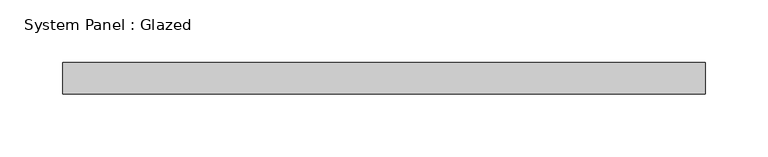
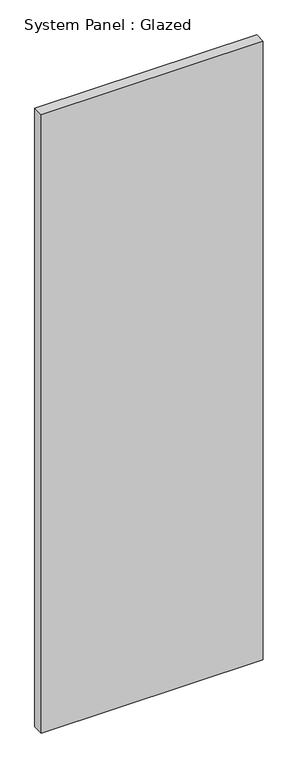
"""IFC4 building model written with IfcOpenShell, lengths in millimetres: plate geometry, System Panel : Glazed."""

from ifc_helpers import new_model, si_unit, origin, origin_with_axes, place, context, project, spatial, polyline, outline, extrude, source, transform, mapped, element, save


def system_panel_glazed_d57a6885(model_context):
    return source(origin(), model_context, "Body", "SweptSolid", [
        extrude(outline(polyline([(257.175, 19.05), (-257.175, 19.05), (-257.175, 44.45), (257.175, 44.45), (257.175, 19.05)])), origin_with_axes(), (0.0, 0.0, 1.0), 1513.1839946),
    ])


if __name__ == "__main__":
    model = new_model("IFC4")
    model_context = context("Model", 3, world=origin())
    ifc_project = project(units=[si_unit("LENGTHUNIT", "METRE", prefix="MILLI")], contexts=[model_context])
    site = spatial("IfcSite", under=ifc_project)
    building = spatial("IfcBuilding", under=site)
    placement = place(None, origin())
    system_panel_glazed_shape = system_panel_glazed_d57a6885(model_context)
    element("IfcPlate", 1, ObjectType="System Panel : Glazed", at=placement, inside=building, context=model_context, shape_type="MappedRepresentation", body=[
        mapped(system_panel_glazed_shape, transform((0.0, 0.0, 0.0), x_axis=(1.0, 0.0, 0.0), y_axis=(0.0, 1.0, 0.0), z_axis=(0.0, 0.0, 1.0))),
    ])
    save(model, "model.ifc")

# Revit data of these elements
# Type "System Panel : Glazed"
#   Construction Type Id = "GSP4R"
#   Analytic Construction = "1/8 in Pilkington single glazing"
#   Visual Light Transmittance = 0.9
#   Solar Heat Gain Coefficient = 0.86
#   Heat Transfer Coefficient (U) = 1.18115 BTU/(h·ft²·°F)
#   Define Thermal Properties by = 1
# Element 1 (IfcPlate, "System Panel : Glazed")
#   Materials on its faces: "Glass"
# Materials
#   "Glass": class "Glass", colour RGB 0 128 192, transparency 0.75, Description = "Soda Lime Glass", Cost = 0
